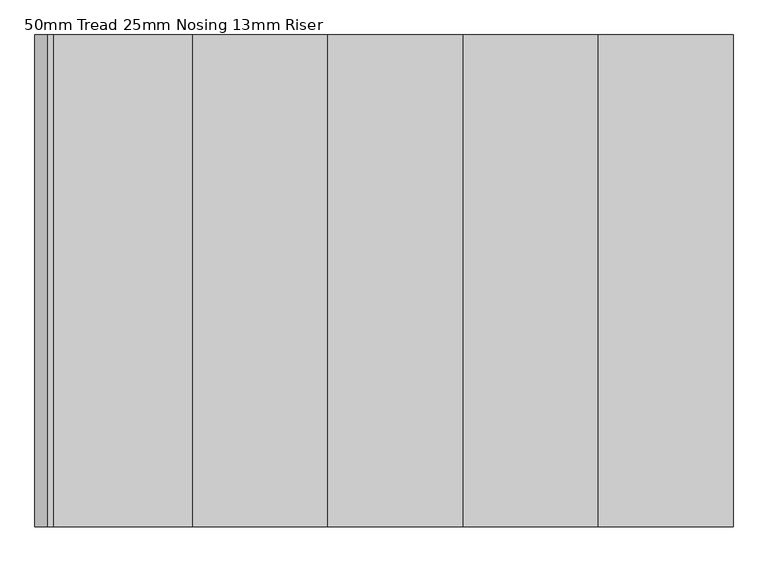
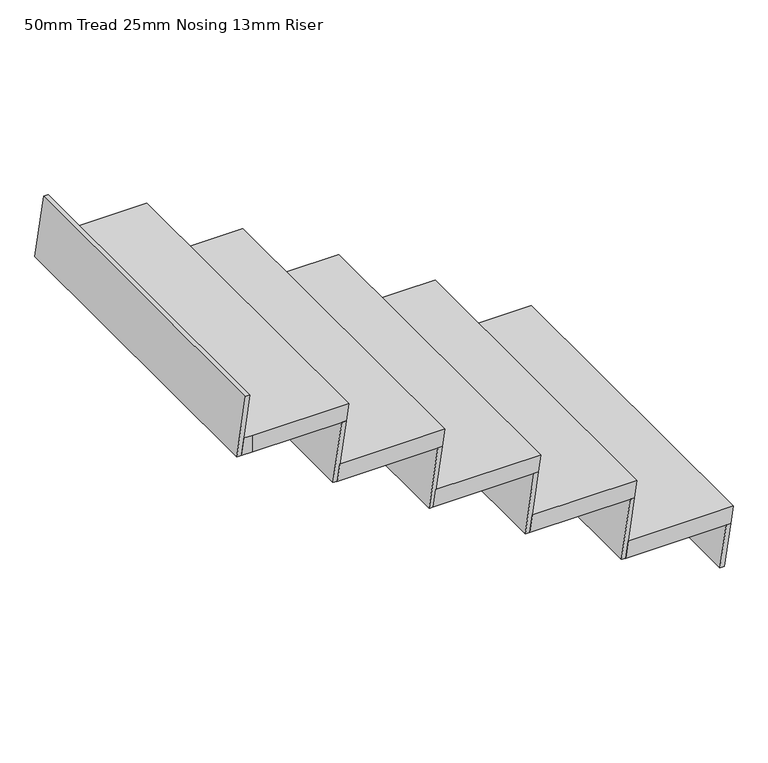
"""IFC4 building model written with IfcOpenShell, lengths in millimetres: stair flight geometry, 50mm Tread 25mm Nosing 13mm Riser."""

from ifc_helpers import new_model, si_unit, origin, place, context, project, spatial, faceted_brep, source, transform, mapped, element, save


def stair_flight_50mm_tread_25mm_nosing_13mm_riser_1fd5534d(model_context):
    return source(origin(), model_context, "Body", "Brep", [
        faceted_brep([(-10476.2529994, 5709.8660835, 173.9130435), (-10483.4404994, 5709.8660835, 123.9130435), (-10483.4404994, 4709.8403022, 123.9130435), (-10476.2529994, 4709.8403022, 173.9130435), (-10176.2529994, 4709.8403022, 173.9130435), (-10176.2529994, 5709.8660835, 173.9130435), (-10183.4404994, 5709.8660835, 123.9130435), (-10183.4404994, 4709.8403022, 123.9130435)], [[[0, 1, 2, 3]], [[3, 4, 5, 0]], [[2, 1, 6, 7]], [[4, 3, 2, 7]], [[0, 5, 6, 1]], [[5, 4, 7, 6]]]),
        faceted_brep([(-10183.4404994, 5709.8660835, 123.9130435), (-10201.2529994, 5709.8660835, 0.0), (-10213.8814894, 5709.8660835, 0.0), (-10196.0689894, 5709.8660835, 123.9130435), (-10183.4404994, 4709.8403022, 123.9130435), (-10196.0689894, 4709.8403022, 123.9130435), (-10213.8814894, 4709.8403022, 0.0), (-10201.2529994, 4709.8403022, 0.0)], [[[0, 1, 2, 3]], [[4, 5, 6, 7]], [[1, 0, 4, 7]], [[2, 1, 7, 6]], [[3, 2, 6, 5]], [[0, 3, 5, 4]]]),
        faceted_brep([(-10458.4404994, 5709.8660835, 297.826087), (-10483.4404994, 5709.8660835, 123.9130435), (-10496.0689894, 5709.8660835, 123.9130435), (-10471.0689894, 5709.8660835, 297.826087), (-10458.4404994, 4709.8403022, 297.826087), (-10471.0689894, 4709.8403022, 297.826087), (-10496.0689894, 4709.8403022, 123.9130435), (-10483.4404994, 4709.8403022, 123.9130435)], [[[0, 1, 2, 3]], [[4, 5, 6, 7]], [[1, 0, 4, 7]], [[2, 1, 7, 6]], [[3, 2, 6, 5]], [[0, 3, 5, 4]]]),
        faceted_brep([(-10751.2529994, 4709.8403022, 347.826087), (-10451.2529994, 4709.8403022, 347.826087), (-10451.2529994, 5709.8660835, 347.826087), (-10751.2529994, 5709.8660835, 347.826087), (-10758.4404994, 4709.8403022, 297.826087), (-10758.4404994, 5709.8660835, 297.826087), (-10458.4404994, 5709.8660835, 297.826087), (-10458.4404994, 4709.8403022, 297.826087)], [[[0, 1, 2, 3]], [[4, 5, 6, 7]], [[1, 0, 4, 7]], [[3, 2, 6, 5]], [[3, 5, 4, 0]], [[2, 1, 7, 6]]]),
        faceted_brep([(-10733.4404994, 5709.8660835, 471.7391304), (-10758.4404994, 5709.8660835, 297.826087), (-10771.0689894, 5709.8660835, 297.826087), (-10746.0689894, 5709.8660835, 471.7391304), (-10733.4404994, 4709.8403022, 471.7391304), (-10746.0689894, 4709.8403022, 471.7391304), (-10771.0689894, 4709.8403022, 297.826087), (-10758.4404994, 4709.8403022, 297.826087)], [[[0, 1, 2, 3]], [[4, 5, 6, 7]], [[1, 0, 4, 7]], [[2, 1, 7, 6]], [[3, 2, 6, 5]], [[0, 3, 5, 4]]]),
        faceted_brep([(-11026.2529994, 4709.8403022, 521.7391304), (-10726.2529994, 4709.8403022, 521.7391304), (-10726.2529994, 5709.8660835, 521.7391304), (-11026.2529994, 5709.8660835, 521.7391304), (-11033.4404994, 4709.8403022, 471.7391304), (-11033.4404994, 5709.8660835, 471.7391304), (-10733.4404994, 5709.8660835, 471.7391304), (-10733.4404994, 4709.8403022, 471.7391304)], [[[0, 1, 2, 3]], [[4, 5, 6, 7]], [[1, 0, 4, 7]], [[3, 2, 6, 5]], [[3, 5, 4, 0]], [[2, 1, 7, 6]]]),
        faceted_brep([(-11008.4404994, 5709.8660835, 645.6521739), (-11033.4404994, 5709.8660835, 471.7391304), (-11046.0689894, 5709.8660835, 471.7391304), (-11021.0689894, 5709.8660835, 645.6521739), (-11008.4404994, 4709.8403022, 645.6521739), (-11021.0689894, 4709.8403022, 645.6521739), (-11046.0689894, 4709.8403022, 471.7391304), (-11033.4404994, 4709.8403022, 471.7391304)], [[[0, 1, 2, 3]], [[4, 5, 6, 7]], [[1, 0, 4, 7]], [[2, 1, 7, 6]], [[3, 2, 6, 5]], [[0, 3, 5, 4]]]),
        faceted_brep([(-11301.2529994, 4709.8403022, 695.6521739), (-11001.2529994, 4709.8403022, 695.6521739), (-11001.2529994, 5709.8660835, 695.6521739), (-11301.2529994, 5709.8660835, 695.6521739), (-11308.4404994, 4709.8403022, 645.6521739), (-11308.4404994, 5709.8660835, 645.6521739), (-11008.4404994, 5709.8660835, 645.6521739), (-11008.4404994, 4709.8403022, 645.6521739)], [[[0, 1, 2, 3]], [[4, 5, 6, 7]], [[1, 0, 4, 7]], [[3, 2, 6, 5]], [[3, 5, 4, 0]], [[2, 1, 7, 6]]]),
        faceted_brep([(-11558.4404994, 5709.8660835, 993.4782609), (-11583.4404994, 5709.8660835, 819.5652174), (-11596.0689894, 5709.8660835, 819.5652174), (-11571.0689894, 5709.8660835, 993.4782609), (-11558.4404994, 4709.8403022, 993.4782609), (-11571.0689894, 4709.8403022, 993.4782609), (-11596.0689894, 4709.8403022, 819.5652174), (-11583.4404994, 4709.8403022, 819.5652174)], [[[0, 1, 2, 3]], [[4, 5, 6, 7]], [[1, 0, 4, 7]], [[2, 1, 7, 6]], [[3, 2, 6, 5]], [[0, 3, 5, 4]]]),
        faceted_brep([(-11283.4404994, 5709.8660835, 819.5652174), (-11308.4404994, 5709.8660835, 645.6521739), (-11321.0689894, 5709.8660835, 645.6521739), (-11296.0689894, 5709.8660835, 819.5652174), (-11283.4404994, 4709.8403022, 819.5652174), (-11296.0689894, 4709.8403022, 819.5652174), (-11321.0689894, 4709.8403022, 645.6521739), (-11308.4404994, 4709.8403022, 645.6521739)], [[[0, 1, 2, 3]], [[4, 5, 6, 7]], [[1, 0, 4, 7]], [[2, 1, 7, 6]], [[3, 2, 6, 5]], [[0, 3, 5, 4]]]),
        faceted_brep([(-11576.2529994, 4709.8403022, 869.5652174), (-11551.2529994, 4709.8403022, 869.5652174), (-11276.2529994, 4709.8403022, 869.5652174), (-11276.2529994, 5709.8660835, 869.5652174), (-11551.2529994, 5709.8660835, 869.5652174), (-11576.2529994, 5709.8660835, 869.5652174), (-11583.4404994, 4709.8403022, 819.5652174), (-11583.4404994, 5709.8660835, 819.5652174), (-11551.2529994, 5709.8660835, 819.5652174), (-11283.4404994, 5709.8660835, 819.5652174), (-11283.4404994, 4709.8403022, 819.5652174), (-11551.2529994, 4709.8403022, 819.5652174)], [[[0, 1, 2, 3, 4, 5]], [[6, 7, 8, 9, 10, 11]], [[1, 0, 6, 11]], [[2, 1, 11, 10]], [[4, 3, 9, 8]], [[5, 7, 6, 0]], [[3, 2, 10, 9]], [[5, 4, 8, 7]]]),
    ])


if __name__ == "__main__":
    model = new_model("IFC4")
    model_context = context("Model", 3, world=origin())
    ifc_project = project(units=[si_unit("LENGTHUNIT", "METRE", prefix="MILLI")], contexts=[model_context])
    site = spatial("IfcSite", under=ifc_project)
    building = spatial("IfcBuilding", under=site)
    placement = place(None, origin())
    stair_flight_50mm_tread_25mm_nosing_13mm_riser_shape = stair_flight_50mm_tread_25mm_nosing_13mm_riser_1fd5534d(model_context)
    element("IfcStairFlight", 1, ObjectType="50mm Tread 25mm Nosing 13mm Riser", at=placement, inside=building, context=model_context, shape_type="MappedRepresentation", body=[
        mapped(stair_flight_50mm_tread_25mm_nosing_13mm_riser_shape, transform((0.0, 0.0, 0.0), x_axis=(1.0, 0.0, 0.0), y_axis=(0.0, 1.0, 0.0), z_axis=(0.0, 0.0, 1.0))),
    ])
    save(model, "model.ifc")
